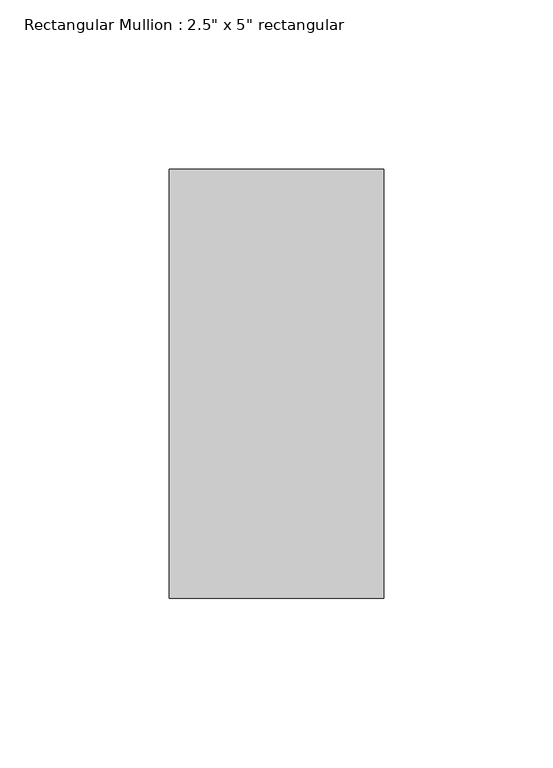
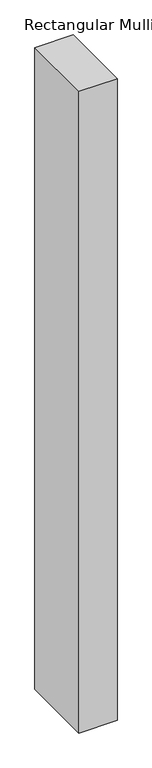
"""IFC4 building model written with IfcOpenShell, lengths in millimetres: member geometry."""

from ifc_helpers import new_model, si_unit, frame, origin, place, context, project, spatial, polyline, outline, extrude, source, transform, mapped, element, save


def member_a08f6adc(model_context):
    return source(origin(), model_context, "Body", "SweptSolid", [
        extrude(outline(polyline([(0.0, 63.5), (0.0, -63.5), (-63.5, -63.5), (-63.5, 63.5), (0.0, 63.5)])), frame((0.0, 0.0, -1130.3), z_axis=(0.0, 0.0, 1.0), x_axis=(1.0, 0.0, 0.0)), (0.0, 0.0, 1.0), 1130.3),
    ])


if __name__ == "__main__":
    model = new_model("IFC4")
    model_context = context("Model", 3, world=origin())
    ifc_project = project(units=[si_unit("LENGTHUNIT", "METRE", prefix="MILLI")], contexts=[model_context])
    site = spatial("IfcSite", under=ifc_project)
    building = spatial("IfcBuilding", under=site)
    placement = place(None, origin())
    member_shape = member_a08f6adc(model_context)
    element("IfcMember", 1, ObjectType="Rectangular Mullion : 2.5\" x 5\" rectangular", at=placement, inside=building, context=model_context, shape_type="MappedRepresentation", body=[
        mapped(member_shape, transform((0.0, 0.0, 0.0), x_axis=(1.0, 0.0, 0.0), y_axis=(0.0, 1.0, 0.0), z_axis=(0.0, 0.0, 1.0))),
    ])
    save(model, "model.ifc")

# Revit data of these elements
# Type "Rectangular Mullion : 2.5\" x 5\" rectangular"
#   built-in parameter 1007304 = 0.416667 (stored number, unit not read)
#   built-in parameter 1007301 = 0.104167 (stored number, unit not read)
#   built-in parameter 1007300 = 0.104167 (stored number, unit not read)
# Element 1 (IfcMember, "Rectangular Mullion : 2.5\" x 5\" rectangular")
#   Materials on its faces: "Aluminum"
# Materials
#   "Aluminum": class "Metal", colour RGB 247 247 247, transparency 0, Description = "Aluminum 6061", Cost = 0
